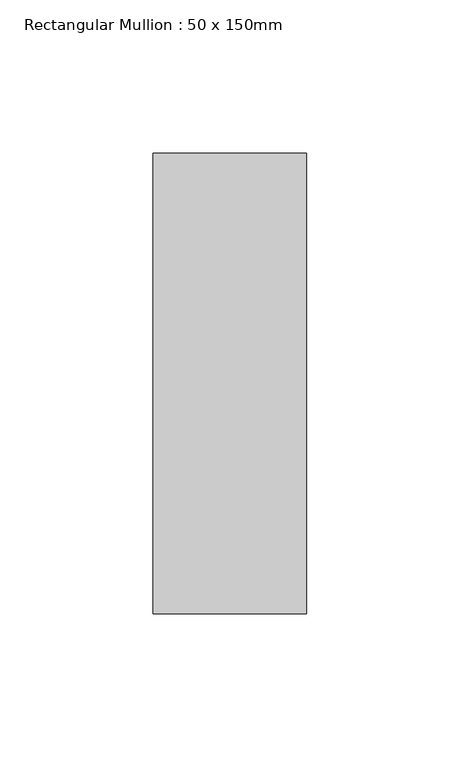
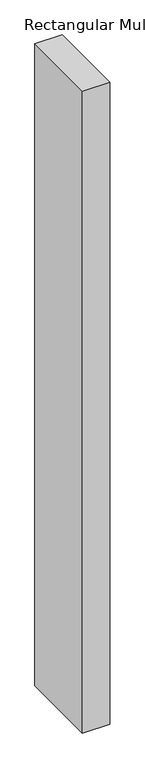
"""IFC4 building model written with IfcOpenShell, lengths in millimetres: member geometry, Rectangular Mullion : 50 x 150mm."""

from ifc_helpers import new_model, si_unit, frame, origin, place, context, project, spatial, polyline, outline, extrude, source, transform, mapped, element, save


def rectangular_mullion_50_x_150mm_c6e312d8(model_context):
    return source(origin(), model_context, "Body", "SweptSolid", [
        extrude(outline(polyline([(0.0, 75.0), (0.0, -75.0), (-50.0, -75.0), (-50.0, 75.0), (0.0, 75.0)])), frame((0.0, 0.0, -1237.5000002), z_axis=(0.0, 0.0, 1.0), x_axis=(1.0, 0.0, 0.0)), (0.0, 0.0, 1.0), 1237.5000002),
    ])


if __name__ == "__main__":
    model = new_model("IFC4")
    model_context = context("Model", 3, world=origin())
    ifc_project = project(units=[si_unit("LENGTHUNIT", "METRE", prefix="MILLI")], contexts=[model_context])
    site = spatial("IfcSite", under=ifc_project)
    building = spatial("IfcBuilding", under=site)
    placement = place(None, origin())
    rectangular_mullion_50_x_150mm_shape = rectangular_mullion_50_x_150mm_c6e312d8(model_context)
    element("IfcMember", 1, ObjectType="Rectangular Mullion : 50 x 150mm", at=placement, inside=building, context=model_context, shape_type="MappedRepresentation", body=[
        mapped(rectangular_mullion_50_x_150mm_shape, transform((0.0, 0.0, 0.0), x_axis=(1.0, 0.0, 0.0), y_axis=(0.0, 1.0, 0.0), z_axis=(0.0, 0.0, 1.0))),
    ])
    save(model, "model.ifc")

# Revit data of these elements
# Type "Rectangular Mullion : 50 x 150mm"
#   built-in parameter 1007304 = 0.492126 (stored number, unit not read)
#   built-in parameter 1007301 = 0.082021 (stored number, unit not read)
#   built-in parameter 1007300 = 0.082021 (stored number, unit not read)
# Element 1 (IfcMember, "Rectangular Mullion : 50 x 150mm")
#   Materials on its faces: "Aluminium"
# Materials
#   "Aluminium": class "Metal", colour RGB 247 247 247, transparency 0, Description = "Aluminium 6061", Cost = 0
